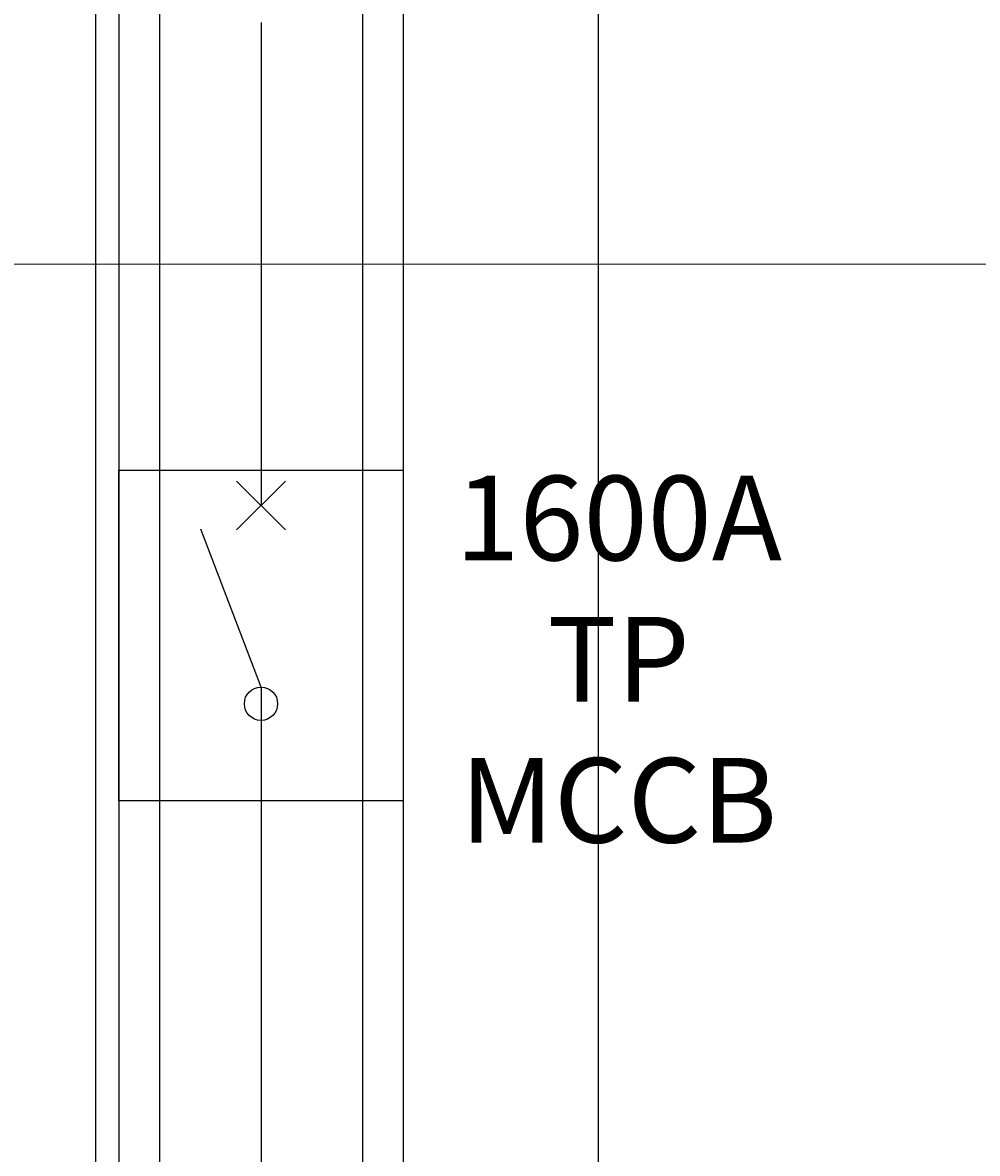
# Model space of a CAD drawing. Units: inches. Extents: x 412 to 584, y 208 to 437.
# Tile 12 of 28: x 494 to 516, y 288 to 315. Entities that reach past the tile are written whole.
import ezdxf

# ---------------------------------------------------------------- set-up
doc = ezdxf.new("R2010")
doc.units = ezdxf.units.IN
doc.header["$MEASUREMENT"] = 0
for name, color, linetype, lineweight in [('A-ANNO-DIMS', 2, 'Continuous', 18), ('E-ANNO-TEXT', 7, 'Continuous', 18), ('E-ENCL', 8, 'Continuous', 18), ('E-POWR-EQPM', 3, 'Continuous', 25)]:
    doc.layers.add(name, color=color, linetype=linetype, lineweight=lineweight)
doc.styles.get("Standard").update_dxf_attribs({"font": 'arial.ttf'})
doc.dimstyles.get("Standard").update_dxf_attribs({"dimtxt": 0.18, "dimasz": 0.18, "dimexe": 0.18, "dimexo": 0.0625, "dimgap": 0.09, "dimtad": 0, "dimtih": 1, "dimtoh": 1, "dimdec": 4, "dimzin": 0, "dimdsep": 46, "dimtxsty": 'Standard', "dimcen": 0.09, "dimadec": 0, "dimazin": 0, "dimtfac": 1, "dimtdec": 4, "dimtofl": 0, "dimtmove": 0, "dimatfit": 3, "dimfxl": 1, "dimtolj": 1, "dimtzin": 0, "dimarcsym": 0})

# ---------------------------------------------------------------- blocks, each defined once
blk = doc.blocks.new('*U5')
blk.add_line((-0.288, 0.288), (0.288, -0.288))
blk = doc.blocks.new('*U6')
at = {"layer": 'E-POWR-EQPM', "color": 0, "linetype": 'ByBlock', "lineweight": -2, "transparency": 16777216}
for p, rotation in [((224.177, 56.28), 180), ((224.754, 56.28), 90), ((224.177, 55.703), 269.9999999999999)]:
    blk.add_blockref('*U5', p, dxfattribs=dict(at, rotation=rotation))
blk.add_blockref('*U5', (224.754, 55.703), dxfattribs=at)
blk = doc.blocks.new('*D17')
at = {"layer": 'A-ANNO-DIMS', "color": 0, "lineweight": -2, "transparency": 16777216}
for p, q in [((497.715, 426.185), (583.674, 426.185)), ((583.494, 426.005), (583.494, 323.031)), ((583.494, 219.693), (583.494, 322.667)), ((550.198, 219.513), (583.674, 219.513))]:
    blk.add_line(p, q, dxfattribs=at)
at = {"layer": 'A-ANNO-DIMS', "color": 0, "transparency": 16777216}
for points in [[(583.464, 426.005), (583.524, 426.005), (583.494, 426.185)], [(583.464, 219.693), (583.524, 219.693), (583.494, 219.513)]]:
    blk.add_solid(points, dxfattribs=at)
at = {"layer": 'Defpoints', "color": 0, "transparency": 16777216}
for p in [(497.652, 426.185), (550.135, 219.513), (583.494, 219.513)]:
    blk.add_point(p, dxfattribs=at)
at = {"layer": 'A-ANNO-DIMS', "color": 0, "transparency": 16777216, "insert": (583.494, 322.849), "char_height": 0.18, "attachment_point": 5}
blk.add_mtext('\\A1;206.67', dxfattribs=at)
blk = doc.blocks.new('*D26')
at = {"layer": 'A-ANNO-DIMS', "color": 0, "lineweight": -2, "transparency": 16777216}
for p, q in [((499.225, 321.294), (412.276, 321.294)), ((412.456, 321.114), (412.456, 315.518)), ((412.456, 309.557), (412.456, 315.154)), ((423.494, 309.377), (412.276, 309.377))]:
    blk.add_line(p, q, dxfattribs=at)
at = {"layer": 'A-ANNO-DIMS', "color": 0, "transparency": 16777216}
for points in [[(412.426, 321.114), (412.486, 321.114), (412.456, 321.294)], [(412.426, 309.557), (412.486, 309.557), (412.456, 309.377)]]:
    blk.add_solid(points, dxfattribs=at)
at = {"layer": 'Defpoints', "color": 0, "transparency": 16777216}
for p in [(499.288, 321.294), (412.456, 309.377), (423.556, 309.377)]:
    blk.add_point(p, dxfattribs=at)
at = {"layer": 'A-ANNO-DIMS', "color": 0, "transparency": 16777216, "insert": (412.456, 315.336), "char_height": 0.18, "attachment_point": 5}
blk.add_mtext('\\A1;11.917', dxfattribs=at)
blk = doc.blocks.new('*D28')
at = {"layer": 'A-ANNO-DIMS', "color": 0, "lineweight": -2, "transparency": 16777216}
for p, q in [((450.562, 256.635), (450.562, 437.465)), ((450.742, 437.285), (502.724, 437.285)), ((555.616, 437.285), (503.634, 437.285)), ((555.796, 256.635), (555.796, 437.465))]:
    blk.add_line(p, q, dxfattribs=at)
at = {"layer": 'A-ANNO-DIMS', "color": 0, "transparency": 16777216}
for points in [[(450.742, 437.315), (450.742, 437.255), (450.562, 437.285)], [(555.616, 437.315), (555.616, 437.255), (555.796, 437.285)]]:
    blk.add_solid(points, dxfattribs=at)
at = {"layer": 'Defpoints', "color": 0, "transparency": 16777216}
for p in [(555.796, 437.285), (450.562, 256.573), (555.796, 256.573)]:
    blk.add_point(p, dxfattribs=at)
at = {"layer": 'A-ANNO-DIMS', "color": 0, "transparency": 16777216, "insert": (503.179, 437.285), "char_height": 0.18, "attachment_point": 5}
blk.add_mtext('\\A1;105.23', dxfattribs=at)
blk = doc.blocks.new('*D29')
at = {"layer": 'A-ANNO-DIMS', "color": 0, "lineweight": -2, "transparency": 16777216}
for p, q in [((495.927, 378.924), (495.927, 208.233)), ((502.649, 378.924), (502.649, 208.233)), ((496.107, 208.413), (498.895, 208.413)), ((502.469, 208.413), (499.681, 208.413))]:
    blk.add_line(p, q, dxfattribs=at)
at = {"layer": 'A-ANNO-DIMS', "color": 0, "transparency": 16777216}
for points in [[(496.107, 208.443), (496.107, 208.383), (495.927, 208.413)], [(502.469, 208.443), (502.469, 208.383), (502.649, 208.413)]]:
    blk.add_solid(points, dxfattribs=at)
at = {"layer": 'Defpoints', "color": 0, "transparency": 16777216}
for p in [(495.927, 378.987), (502.649, 378.987), (502.649, 208.413)]:
    blk.add_point(p, dxfattribs=at)
at = {"layer": 'A-ANNO-DIMS', "color": 0, "transparency": 16777216, "insert": (499.288, 208.413), "char_height": 0.18, "attachment_point": 5}
blk.add_mtext('\\A1;6.722', dxfattribs=at)
blk = doc.blocks.new('*D31')
at = {"layer": 'A-ANNO-DIMS', "color": 0, "lineweight": -2, "transparency": 16777216}
for p, q in [((495.375, 405.385), (495.375, 208.233)), ((507.254, 405.385), (507.254, 208.233)), ((495.555, 208.413), (500.929, 208.413)), ((507.074, 208.413), (501.7, 208.413))]:
    blk.add_line(p, q, dxfattribs=at)
at = {"layer": 'A-ANNO-DIMS', "color": 0, "transparency": 16777216}
for points in [[(495.555, 208.443), (495.555, 208.383), (495.375, 208.413)], [(507.074, 208.443), (507.074, 208.383), (507.254, 208.413)]]:
    blk.add_solid(points, dxfattribs=at)
at = {"layer": 'Defpoints', "color": 0, "transparency": 16777216}
for p in [(495.375, 405.448), (507.254, 405.448), (507.254, 208.413)]:
    blk.add_point(p, dxfattribs=at)
at = {"layer": 'A-ANNO-DIMS', "color": 0, "transparency": 16777216, "insert": (501.314, 208.413), "char_height": 0.18, "attachment_point": 5}
blk.add_mtext('\\A1;11.88', dxfattribs=at)
blk = doc.blocks.new('*D39')
at = {"layer": 'A-ANNO-DIMS', "color": 0, "lineweight": -2, "transparency": 16777216}
for p, q in [((496.891, 346.914), (496.891, 208.233)), ((501.685, 346.914), (501.685, 208.233)), ((497.071, 208.413), (498.891, 208.413)), ((501.505, 208.413), (499.685, 208.413))]:
    blk.add_line(p, q, dxfattribs=at)
at = {"layer": 'A-ANNO-DIMS', "color": 0, "transparency": 16777216}
for points in [[(497.071, 208.443), (497.071, 208.383), (496.891, 208.413)], [(501.505, 208.443), (501.505, 208.383), (501.685, 208.413)]]:
    blk.add_solid(points, dxfattribs=at)
at = {"layer": 'Defpoints', "color": 0, "transparency": 16777216}
for p in [(496.891, 346.977), (501.685, 346.977), (501.685, 208.413)]:
    blk.add_point(p, dxfattribs=at)
at = {"layer": 'A-ANNO-DIMS', "color": 0, "transparency": 16777216, "insert": (499.288, 208.413), "char_height": 0.18, "attachment_point": 5}
blk.add_mtext('\\A1;4.794', dxfattribs=at)

msp = doc.modelspace()

# ---------------------------------------------------------------- linework, layer by layer
at = {"layer": 'E-ENCL'}
msp.add_lwpolyline([(423.5562, 309.3773), (572.3937, 309.3773), (572.3937, 225.5881), (423.5562, 225.5881)], close=True, dxfattribs=at)
at = {"layer": 'E-POWR-EQPM'}
for p, q in [((499.2878, 315.082), (499.2878, 303.6727)), ((499.2878, 299.3838), (497.8672, 303.1182)), ((499.2878, 299.3838), (499.2878, 284.4906))]:
    msp.add_line(p, q, dxfattribs=at)
msp.add_lwpolyline([(495.9268, 304.5061), (502.6489, 304.5061), (502.6489, 296.6994), (495.9268, 296.6994)], close=True, dxfattribs=at)
msp.add_circle((499.2878, 298.9904), 0.3935, dxfattribs=at)

# ---------------------------------------------------------------- block references
msp.add_blockref('*U6', (274.8225, 247.6811), dxfattribs=at)

# ---------------------------------------------------------------- texts
at = {"layer": 'E-ANNO-TEXT', "insert": (499.4044, 304.3783), "char_height": 2, "attachment_point": 1}
msp.add_mtext_dynamic_manual_height_columns('\\pxqc;1600A\\PTP\\PMCCB', width=16.663738, gutter_width=1, heights=[13.9227], dxfattribs=at)

# ---------------------------------------------------------------- dimensions: what is measured, and where the dimension line sits
at = {"layer": 'A-ANNO-DIMS'}
for base, p1, p2, override, picture, middle in [((555.7959, 437.2847), (450.562, 256.5729), (555.7959, 256.5729), {"dimdec": 2, "dimlfac": 1, "dimrnd": 0, "dimzin": 0, "dimdsep": 46, "dimlunit": 2}, '*D28', (503.1789, 437.2847)), ((507.2538, 208.4133), (495.3746, 405.448), (507.2538, 405.448), {"dimdec": 2, "dimlfac": 1, "dimrnd": 0, "dimzin": 0, "dimdsep": 46, "dimlunit": 2}, '*D31', (501.3142, 208.4133)), ((502.6489, 208.4133), (495.9268, 378.9867), (502.6489, 378.9867), {"dimdec": 3, "dimlfac": 1, "dimrnd": 0, "dimzin": 0, "dimdsep": 46, "dimlunit": 2}, '*D29', (499.2878, 208.4133)), ((501.6846, 208.4133), (496.891, 346.9765), (501.6846, 346.9765), {"dimdec": 3, "dimlfac": 1, "dimrnd": 0, "dimzin": 0, "dimdsep": 46, "dimlunit": 2}, '*D39', (499.2878, 208.4133))]:
    dim = msp.add_linear_dim(base=base, p1=p1, p2=p2, dimstyle='Standard', override=override, dxfattribs=at)
    dim.commit()
    dim.dimension.update_dxf_attribs({"geometry": picture, "text_midpoint": middle})
for base, p1, p2, override, picture, middle in [((583.4937, 219.5133), (497.6523, 426.1847), (550.1351, 219.5133), {"dimdec": 2, "dimlfac": 1, "dimrnd": 0, "dimzin": 0, "dimdsep": 46, "dimlunit": 2}, '*D17', (583.4937, 322.849)), ((412.4562, 309.3773), (499.2878, 321.2941), (423.5562, 309.3773), {"dimdec": 3, "dimlfac": 1, "dimrnd": 0, "dimzin": 0, "dimdsep": 46, "dimlunit": 2}, '*D26', (412.4562, 315.3357))]:
    dim = msp.add_linear_dim(base=base, p1=p1, p2=p2, angle=90, dimstyle='Standard', override=override, dxfattribs=at)
    dim.commit()
    dim.dimension.update_dxf_attribs({"geometry": picture, "text_midpoint": middle})

doc.saveas('drawing.dxf')
